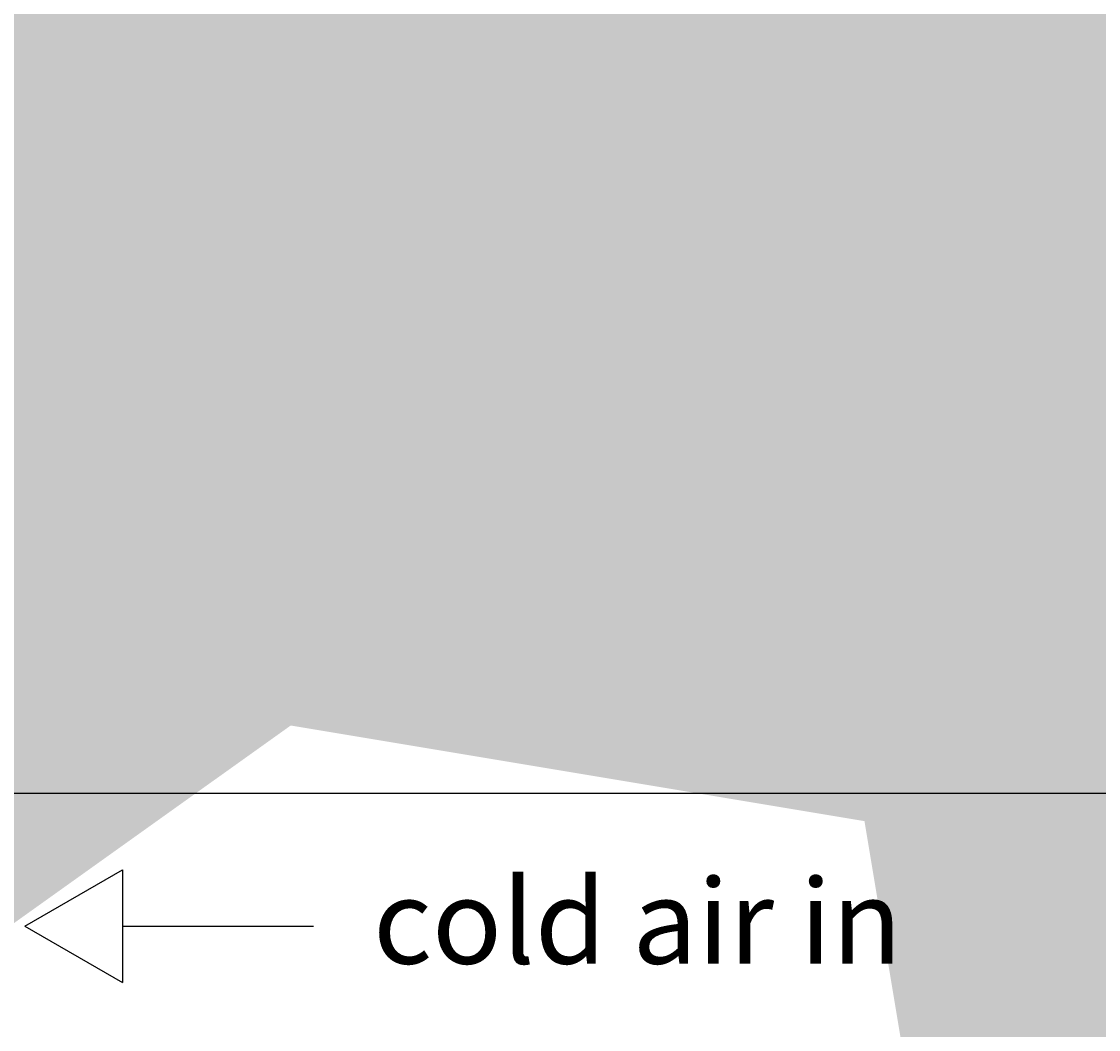
# Model space of a CAD drawing. Units: millimetres. Extents: x -22994 to 29398, y -19990 to 20176.
# Tile 121 of 135: x 245 to 296, y 165 to 213. Entities that reach past the tile are written whole.
import ezdxf

# ---------------------------------------------------------------- set-up
doc = ezdxf.new("R2010")
doc.units = ezdxf.units.MM
doc.header["$MEASUREMENT"] = 0
for name, color, linetype, lineweight in [('M-ANNO-SYMB', 7, 'Continuous', 25), ('M-ANNO-TEXT', 7, 'Continuous', 25), ('M-DIMS', 2, 'Continuous', 18)]:
    doc.layers.add(name, color=color, linetype=linetype, lineweight=lineweight)
doc.styles.get("Standard").update_dxf_attribs({"font": 'arial.ttf'})
doc.dimstyles.get("Standard").update_dxf_attribs({"dimtxt": 0.18, "dimasz": 10000, "dimexe": 0.18, "dimexo": 0.0625, "dimgap": 0.09, "dimtad": 0, "dimtih": 1, "dimtoh": 1, "dimdec": 0, "dimzin": 0, "dimdsep": 46, "dimtxsty": 'Standard', "dimcen": 0.09, "dimadec": 0, "dimazin": 0, "dimtfac": 1, "dimtdec": 0, "dimtofl": 0, "dimtmove": 0, "dimatfit": 3, "dimfxl": 1, "dimtolj": 1, "dimtzin": 0, "dimlwd": 30, "dimarcsym": 0})

# ---------------------------------------------------------------- blocks, each defined once
blk = doc.blocks.new('ARROW-FLOW')
for p, q in [((4.609, 5.322), (0, 2.661)), ((4.609, 5.322), (4.609, 0)), ((4.609, 0), (0, 2.661))]:
    blk.add_line(p, q)
blk = doc.blocks.new('*D2')
at = {"layer": 'Defpoints', "color": 0, "transparency": 16777216}
for p in [(6.677, 10.271), (290.852, 10.271), (290.852, -5.079)]:
    blk.add_point(p, dxfattribs=at)
at = {"layer": 'M-DIMS', "color": 0, "lineweight": -2, "transparency": 16777216}
for p, q in [((6.677, 10.209), (6.677, -5.259)), ((290.852, 10.209), (290.852, -5.259))]:
    blk.add_line(p, q, dxfattribs=at)
at = {"layer": 'M-DIMS', "color": 0, "lineweight": 30, "transparency": 16777216}
for p, q in [((-9993.323, -5.079), (-19993.323, -5.079)), ((10290.852, -5.079), (20290.852, -5.079))]:
    blk.add_line(p, q, dxfattribs=at)
at = {"layer": 'M-DIMS', "color": 0, "transparency": 16777216}
for points in [[(-9993.323, 1661.588), (-9993.323, -1671.745), (6.677, -5.079)], [(10290.852, 1661.588), (10290.852, -1671.745), (290.852, -5.079)]]:
    blk.add_solid(points, dxfattribs=at)
at = {"layer": 'M-DIMS', "color": 0, "transparency": 16777216, "insert": (148.765, -5.079), "char_height": 0.18, "attachment_point": 5}
blk.add_mtext('\\A1;284.2', dxfattribs=at)
blk = doc.blocks.new('*D3')
at = {"layer": 'Defpoints', "color": 0, "transparency": 16777216}
for p in [(110.265, 204.165), (110.265, 176.366), (95.833, 127.967)]:
    blk.add_point(p, dxfattribs=at)
at = {"layer": 'M-DIMS', "color": 0, "lineweight": 30, "transparency": 16777216}
for p, q in [((-9904.167, 204.165), (-19904.167, 204.165)), ((10110.265, 204.165), (20110.265, 204.165))]:
    blk.add_line(p, q, dxfattribs=at)
at = {"layer": 'M-DIMS', "color": 0, "lineweight": -2, "transparency": 16777216}
for p, q in [((95.833, 128.03), (95.833, 204.345)), ((110.265, 176.429), (110.265, 204.345))]:
    blk.add_line(p, q, dxfattribs=at)
at = {"layer": 'M-DIMS', "color": 0, "transparency": 16777216}
for points in [[(-9904.167, 1870.832), (-9904.167, -1462.501), (95.833, 204.165)], [(10110.265, 1870.832), (10110.265, -1462.501), (110.265, 204.165)]]:
    blk.add_solid(points, dxfattribs=at)
at = {"layer": 'M-DIMS', "color": 0, "transparency": 16777216, "insert": (103.049, 204.165), "char_height": 0.18, "attachment_point": 5}
blk.add_mtext('\\A1;14.432', dxfattribs=at)
blk = doc.blocks.new('*D4')
at = {"layer": 'Defpoints', "color": 0, "transparency": 16777216}
for p in [(116.265, 204.165), (110.265, 176.366), (116.265, 176.366)]:
    blk.add_point(p, dxfattribs=at)
at = {"layer": 'M-DIMS', "color": 0, "lineweight": 30, "transparency": 16777216}
for p, q in [((-9889.735, 204.165), (-19889.735, 204.165)), ((10116.265, 204.165), (20116.265, 204.165))]:
    blk.add_line(p, q, dxfattribs=at)
at = {"layer": 'M-DIMS', "color": 0, "lineweight": -2, "transparency": 16777216}
for p, q in [((110.265, 176.429), (110.265, 204.345)), ((116.265, 176.429), (116.265, 204.345))]:
    blk.add_line(p, q, dxfattribs=at)
at = {"layer": 'M-DIMS', "color": 0, "transparency": 16777216}
for points in [[(-9889.735, 1870.832), (-9889.735, -1462.501), (110.265, 204.165)], [(10116.265, 1870.832), (10116.265, -1462.501), (116.265, 204.165)]]:
    blk.add_solid(points, dxfattribs=at)
at = {"layer": 'M-DIMS', "color": 0, "transparency": 16777216, "insert": (113.265, 204.165), "char_height": 0.18, "attachment_point": 5}
blk.add_mtext('\\A1;6', dxfattribs=at)
blk = doc.blocks.new('*D5')
at = {"layer": 'Defpoints', "color": 0, "transparency": 16777216}
for p in [(181.265, 204.165), (116.265, 176.366), (181.265, 176.366)]:
    blk.add_point(p, dxfattribs=at)
at = {"layer": 'M-DIMS', "color": 0, "lineweight": 30, "transparency": 16777216}
for p, q in [((-9883.735, 204.165), (-19883.735, 204.165)), ((10181.265, 204.165), (20181.265, 204.165))]:
    blk.add_line(p, q, dxfattribs=at)
at = {"layer": 'M-DIMS', "color": 0, "lineweight": -2, "transparency": 16777216}
for p, q in [((116.265, 176.429), (116.265, 204.345)), ((181.265, 176.429), (181.265, 204.345))]:
    blk.add_line(p, q, dxfattribs=at)
at = {"layer": 'M-DIMS', "color": 0, "transparency": 16777216}
for points in [[(-9883.735, 1870.832), (-9883.735, -1462.501), (116.265, 204.165)], [(10181.265, 1870.832), (10181.265, -1462.501), (181.265, 204.165)]]:
    blk.add_solid(points, dxfattribs=at)
at = {"layer": 'M-DIMS', "color": 0, "transparency": 16777216, "insert": (148.765, 204.165), "char_height": 0.18, "attachment_point": 5}
blk.add_mtext('\\A1;65', dxfattribs=at)
blk = doc.blocks.new('*D6')
at = {"layer": 'Defpoints', "color": 0, "transparency": 16777216}
for p in [(187.265, 204.165), (181.265, 176.366), (187.265, 176.366)]:
    blk.add_point(p, dxfattribs=at)
at = {"layer": 'M-DIMS', "color": 0, "lineweight": 30, "transparency": 16777216}
for p, q in [((-9818.735, 204.165), (-19818.735, 204.165)), ((10187.265, 204.165), (20187.265, 204.165))]:
    blk.add_line(p, q, dxfattribs=at)
at = {"layer": 'M-DIMS', "color": 0, "lineweight": -2, "transparency": 16777216}
for p, q in [((181.265, 176.429), (181.265, 204.345)), ((187.265, 176.429), (187.265, 204.345))]:
    blk.add_line(p, q, dxfattribs=at)
at = {"layer": 'M-DIMS', "color": 0, "transparency": 16777216}
for points in [[(-9818.735, 1870.832), (-9818.735, -1462.501), (181.265, 204.165)], [(10187.265, 1870.832), (10187.265, -1462.501), (187.265, 204.165)]]:
    blk.add_solid(points, dxfattribs=at)
at = {"layer": 'M-DIMS', "color": 0, "transparency": 16777216, "insert": (184.265, 204.165), "char_height": 0.18, "attachment_point": 5}
blk.add_mtext('\\A1;6', dxfattribs=at)
blk = doc.blocks.new('*D7')
at = {"layer": 'Defpoints', "color": 0, "transparency": 16777216}
for p in [(201.697, 204.165), (187.265, 176.366), (201.697, 127.967)]:
    blk.add_point(p, dxfattribs=at)
at = {"layer": 'M-DIMS', "color": 0, "lineweight": 30, "transparency": 16777216}
for p, q in [((-9812.735, 204.165), (-19812.735, 204.165)), ((10201.697, 204.165), (20201.697, 204.165))]:
    blk.add_line(p, q, dxfattribs=at)
at = {"layer": 'M-DIMS', "color": 0, "lineweight": -2, "transparency": 16777216}
for p, q in [((187.265, 176.429), (187.265, 204.345)), ((201.697, 128.03), (201.697, 204.345))]:
    blk.add_line(p, q, dxfattribs=at)
at = {"layer": 'M-DIMS', "color": 0, "transparency": 16777216}
for points in [[(-9812.735, 1870.832), (-9812.735, -1462.501), (187.265, 204.165)], [(10201.697, 1870.832), (10201.697, -1462.501), (201.697, 204.165)]]:
    blk.add_solid(points, dxfattribs=at)
at = {"layer": 'M-DIMS', "color": 0, "transparency": 16777216, "insert": (194.481, 204.165), "char_height": 0.18, "attachment_point": 5}
blk.add_mtext('\\A1;14.432', dxfattribs=at)
blk = doc.blocks.new('*D8')
at = {"layer": 'Defpoints', "color": 0, "transparency": 16777216}
for p in [(227.648, 204.165), (227.648, 146.73), (201.697, 127.967)]:
    blk.add_point(p, dxfattribs=at)
at = {"layer": 'M-DIMS', "color": 0, "lineweight": 30, "transparency": 16777216}
for p, q in [((-9798.303, 204.165), (-19798.303, 204.165)), ((10227.648, 204.165), (20227.648, 204.165))]:
    blk.add_line(p, q, dxfattribs=at)
at = {"layer": 'M-DIMS', "color": 0, "lineweight": -2, "transparency": 16777216}
for p, q in [((201.697, 128.03), (201.697, 204.345)), ((227.648, 146.792), (227.648, 204.345))]:
    blk.add_line(p, q, dxfattribs=at)
at = {"layer": 'M-DIMS', "color": 0, "transparency": 16777216}
for points in [[(-9798.303, 1870.832), (-9798.303, -1462.501), (201.697, 204.165)], [(10227.648, 1870.832), (10227.648, -1462.501), (227.648, 204.165)]]:
    blk.add_solid(points, dxfattribs=at)
at = {"layer": 'M-DIMS', "color": 0, "transparency": 16777216, "insert": (214.673, 204.165), "char_height": 0.18, "attachment_point": 5}
blk.add_mtext('\\A1;25.95', dxfattribs=at)
blk = doc.blocks.new('*D9')
at = {"layer": 'Defpoints', "color": 0, "transparency": 16777216}
for p in [(187.265, 176.366), (306.202, 176.366), (290.852, 10.271)]:
    blk.add_point(p, dxfattribs=at)
at = {"layer": 'M-DIMS', "color": 0, "lineweight": 30, "transparency": 16777216}
for p, q in [((306.202, 10176.366), (306.202, 20176.366)), ((306.202, -9989.729), (306.202, -19989.729))]:
    blk.add_line(p, q, dxfattribs=at)
at = {"layer": 'M-DIMS', "color": 0, "lineweight": -2, "transparency": 16777216}
for p, q in [((187.327, 176.366), (306.382, 176.366)), ((290.915, 10.271), (306.382, 10.271))]:
    blk.add_line(p, q, dxfattribs=at)
at = {"layer": 'M-DIMS', "color": 0, "transparency": 16777216}
for points in [[(-1360.465, 10176.366), (1972.869, 10176.366), (306.202, 176.366)], [(-1360.465, -9989.729), (1972.869, -9989.729), (306.202, 10.271)]]:
    blk.add_solid(points, dxfattribs=at)
at = {"layer": 'M-DIMS', "color": 0, "transparency": 16777216, "insert": (306.202, 93.319), "char_height": 0.18, "attachment_point": 5}
blk.add_mtext('\\A1;166.1', dxfattribs=at)
blk = doc.blocks.new('*D10')
at = {"layer": 'Defpoints', "color": 0, "transparency": 16777216}
for p in [(125.65, 136.071), (133.346, 136.071), (133.346, -5.079)]:
    blk.add_point(p, dxfattribs=at)
at = {"layer": 'M-DIMS', "color": 0, "lineweight": -2, "transparency": 16777216}
for p, q in [((125.65, 136.009), (125.65, -5.259)), ((133.346, 136.009), (133.346, -5.259))]:
    blk.add_line(p, q, dxfattribs=at)
at = {"layer": 'M-DIMS', "color": 0, "lineweight": 30, "transparency": 16777216}
for p, q in [((-9874.35, -5.079), (-19874.35, -5.079)), ((10133.346, -5.079), (20133.346, -5.079))]:
    blk.add_line(p, q, dxfattribs=at)
at = {"layer": 'M-DIMS', "color": 0, "transparency": 16777216}
for points in [[(-9874.35, 1661.588), (-9874.35, -1671.745), (125.65, -5.079)], [(10133.346, 1661.588), (10133.346, -1671.745), (133.346, -5.079)]]:
    blk.add_solid(points, dxfattribs=at)
at = {"layer": 'M-DIMS', "color": 0, "transparency": 16777216, "insert": (129.498, -5.079), "char_height": 0.18, "attachment_point": 5}
blk.add_mtext('\\A1;7.696', dxfattribs=at)
blk = doc.blocks.new('*D11')
at = {"layer": 'Defpoints', "color": 0, "transparency": 16777216}
for p in [(133.346, 136.071), (135.65, 136.071), (135.65, -5.079)]:
    blk.add_point(p, dxfattribs=at)
at = {"layer": 'M-DIMS', "color": 0, "lineweight": -2, "transparency": 16777216}
for p, q in [((133.346, 136.009), (133.346, -5.259)), ((135.65, 136.009), (135.65, -5.259))]:
    blk.add_line(p, q, dxfattribs=at)
at = {"layer": 'M-DIMS', "color": 0, "lineweight": 30, "transparency": 16777216}
for p, q in [((-9866.654, -5.079), (-19866.654, -5.079)), ((10135.65, -5.079), (20135.65, -5.079))]:
    blk.add_line(p, q, dxfattribs=at)
at = {"layer": 'M-DIMS', "color": 0, "transparency": 16777216}
for points in [[(-9866.654, 1661.588), (-9866.654, -1671.745), (133.346, -5.079)], [(10135.65, 1661.588), (10135.65, -1671.745), (135.65, -5.079)]]:
    blk.add_solid(points, dxfattribs=at)
at = {"layer": 'M-DIMS', "color": 0, "transparency": 16777216, "insert": (134.498, -5.079), "char_height": 0.18, "attachment_point": 5}
blk.add_mtext('\\A1;2.304', dxfattribs=at)
blk = doc.blocks.new('*D12')
at = {"layer": 'Defpoints', "color": 0, "transparency": 16777216}
for p in [(135.65, 136.071), (145.65, 136.071), (145.65, -5.079)]:
    blk.add_point(p, dxfattribs=at)
at = {"layer": 'M-DIMS', "color": 0, "lineweight": -2, "transparency": 16777216}
for p, q in [((135.65, 136.009), (135.65, -5.259)), ((145.65, 136.009), (145.65, -5.259))]:
    blk.add_line(p, q, dxfattribs=at)
at = {"layer": 'M-DIMS', "color": 0, "lineweight": 30, "transparency": 16777216}
for p, q in [((-9864.35, -5.079), (-19864.35, -5.079)), ((10145.65, -5.079), (20145.65, -5.079))]:
    blk.add_line(p, q, dxfattribs=at)
at = {"layer": 'M-DIMS', "color": 0, "transparency": 16777216}
for points in [[(-9864.35, 1661.588), (-9864.35, -1671.745), (135.65, -5.079)], [(10145.65, 1661.588), (10145.65, -1671.745), (145.65, -5.079)]]:
    blk.add_solid(points, dxfattribs=at)
at = {"layer": 'M-DIMS', "color": 0, "transparency": 16777216, "insert": (140.65, -5.079), "char_height": 0.18, "attachment_point": 5}
blk.add_mtext('\\A1;10', dxfattribs=at)
blk = doc.blocks.new('*D13')
at = {"layer": 'Defpoints', "color": 0, "transparency": 16777216}
for p in [(145.65, 136.071), (155.65, 136.071), (155.65, -5.079)]:
    blk.add_point(p, dxfattribs=at)
at = {"layer": 'M-DIMS', "color": 0, "lineweight": -2, "transparency": 16777216}
for p, q in [((145.65, 136.009), (145.65, -5.259)), ((155.65, 136.009), (155.65, -5.259))]:
    blk.add_line(p, q, dxfattribs=at)
at = {"layer": 'M-DIMS', "color": 0, "lineweight": 30, "transparency": 16777216}
for p, q in [((-9854.35, -5.079), (-19854.35, -5.079)), ((10155.65, -5.079), (20155.65, -5.079))]:
    blk.add_line(p, q, dxfattribs=at)
at = {"layer": 'M-DIMS', "color": 0, "transparency": 16777216}
for points in [[(-9854.35, 1661.588), (-9854.35, -1671.745), (145.65, -5.079)], [(10155.65, 1661.588), (10155.65, -1671.745), (155.65, -5.079)]]:
    blk.add_solid(points, dxfattribs=at)
at = {"layer": 'M-DIMS', "color": 0, "transparency": 16777216, "insert": (150.65, -5.079), "char_height": 0.18, "attachment_point": 5}
blk.add_mtext('\\A1;10', dxfattribs=at)
blk = doc.blocks.new('*D14')
at = {"layer": 'Defpoints', "color": 0, "transparency": 16777216}
for p in [(155.65, 136.071), (165.65, 136.071), (165.65, -5.079)]:
    blk.add_point(p, dxfattribs=at)
at = {"layer": 'M-DIMS', "color": 0, "lineweight": -2, "transparency": 16777216}
for p, q in [((155.65, 136.009), (155.65, -5.259)), ((165.65, 136.009), (165.65, -5.259))]:
    blk.add_line(p, q, dxfattribs=at)
at = {"layer": 'M-DIMS', "color": 0, "lineweight": 30, "transparency": 16777216}
for p, q in [((-9844.35, -5.079), (-19844.35, -5.079)), ((10165.65, -5.079), (20165.65, -5.079))]:
    blk.add_line(p, q, dxfattribs=at)
at = {"layer": 'M-DIMS', "color": 0, "transparency": 16777216}
for points in [[(-9844.35, 1661.588), (-9844.35, -1671.745), (155.65, -5.079)], [(10165.65, 1661.588), (10165.65, -1671.745), (165.65, -5.079)]]:
    blk.add_solid(points, dxfattribs=at)
at = {"layer": 'M-DIMS', "color": 0, "transparency": 16777216, "insert": (160.65, -5.079), "char_height": 0.18, "attachment_point": 5}
blk.add_mtext('\\A1;10', dxfattribs=at)
blk = doc.blocks.new('*D15')
at = {"layer": 'Defpoints', "color": 0, "transparency": 16777216}
for p in [(173.346, 154.788), (173.346, 136.071), (306.202, 136.071)]:
    blk.add_point(p, dxfattribs=at)
at = {"layer": 'M-DIMS', "color": 0, "lineweight": 30, "transparency": 16777216}
for p, q in [((306.202, 10154.788), (306.202, 20154.788)), ((306.202, -9863.929), (306.202, -19863.929))]:
    blk.add_line(p, q, dxfattribs=at)
at = {"layer": 'M-DIMS', "color": 0, "lineweight": -2, "transparency": 16777216}
for p, q in [((173.408, 154.788), (306.382, 154.788)), ((173.408, 136.071), (306.382, 136.071))]:
    blk.add_line(p, q, dxfattribs=at)
at = {"layer": 'M-DIMS', "color": 0, "transparency": 16777216}
for points in [[(-1360.465, 10154.788), (1972.869, 10154.788), (306.202, 154.788)], [(-1360.465, -9863.929), (1972.869, -9863.929), (306.202, 136.071)]]:
    blk.add_solid(points, dxfattribs=at)
at = {"layer": 'M-DIMS', "color": 0, "transparency": 16777216, "insert": (306.202, 145.43), "char_height": 0.18, "attachment_point": 5}
blk.add_mtext('\\A1;18.717', dxfattribs=at)
blk = doc.blocks.new('*D16')
at = {"layer": 'Defpoints', "color": 0, "transparency": 16777216}
for p in [(120.17, 204.165), (110.466, 48.035), (120.17, 48.035)]:
    blk.add_point(p, dxfattribs=at)
at = {"layer": 'M-DIMS', "color": 0, "lineweight": 30, "transparency": 16777216}
for p, q in [((-9889.534, 204.165), (-19889.534, 204.165)), ((10120.17, 204.165), (20120.17, 204.165))]:
    blk.add_line(p, q, dxfattribs=at)
at = {"layer": 'M-DIMS', "color": 0, "lineweight": -2, "transparency": 16777216}
for p, q in [((110.466, 48.097), (110.466, 204.345)), ((120.17, 48.097), (120.17, 204.345))]:
    blk.add_line(p, q, dxfattribs=at)
at = {"layer": 'M-DIMS', "color": 0, "transparency": 16777216}
for points in [[(-9889.534, 1870.832), (-9889.534, -1462.501), (110.466, 204.165)], [(10120.17, 1870.832), (10120.17, -1462.501), (120.17, 204.165)]]:
    blk.add_solid(points, dxfattribs=at)
at = {"layer": 'M-DIMS', "color": 0, "transparency": 16777216, "insert": (115.318, 204.165), "char_height": 0.18, "attachment_point": 5}
blk.add_mtext('\\A1;9.704', dxfattribs=at)
blk = doc.blocks.new('*D17')
at = {"layer": 'Defpoints', "color": 0, "transparency": 16777216}
for p in [(126.17, 204.165), (120.17, 48.035), (126.17, 48.035)]:
    blk.add_point(p, dxfattribs=at)
at = {"layer": 'M-DIMS', "color": 0, "lineweight": 30, "transparency": 16777216}
for p, q in [((-9879.83, 204.165), (-19879.83, 204.165)), ((10126.17, 204.165), (20126.17, 204.165))]:
    blk.add_line(p, q, dxfattribs=at)
at = {"layer": 'M-DIMS', "color": 0, "lineweight": -2, "transparency": 16777216}
for p, q in [((120.17, 48.097), (120.17, 204.345)), ((126.17, 48.097), (126.17, 204.345))]:
    blk.add_line(p, q, dxfattribs=at)
at = {"layer": 'M-DIMS', "color": 0, "transparency": 16777216}
for points in [[(-9879.83, 1870.832), (-9879.83, -1462.501), (120.17, 204.165)], [(10126.17, 1870.832), (10126.17, -1462.501), (126.17, 204.165)]]:
    blk.add_solid(points, dxfattribs=at)
at = {"layer": 'M-DIMS', "color": 0, "transparency": 16777216, "insert": (123.17, 204.165), "char_height": 0.18, "attachment_point": 5}
blk.add_mtext('\\A1;6', dxfattribs=at)
blk = doc.blocks.new('*D18')
at = {"layer": 'Defpoints', "color": 0, "transparency": 16777216}
for p in [(132.17, 204.165), (126.17, 48.035), (132.17, 48.035)]:
    blk.add_point(p, dxfattribs=at)
at = {"layer": 'M-DIMS', "color": 0, "lineweight": 30, "transparency": 16777216}
for p, q in [((-9873.83, 204.165), (-19873.83, 204.165)), ((10132.17, 204.165), (20132.17, 204.165))]:
    blk.add_line(p, q, dxfattribs=at)
at = {"layer": 'M-DIMS', "color": 0, "lineweight": -2, "transparency": 16777216}
for p, q in [((126.17, 48.097), (126.17, 204.345)), ((132.17, 48.097), (132.17, 204.345))]:
    blk.add_line(p, q, dxfattribs=at)
at = {"layer": 'M-DIMS', "color": 0, "transparency": 16777216}
for points in [[(-9873.83, 1870.832), (-9873.83, -1462.501), (126.17, 204.165)], [(10132.17, 1870.832), (10132.17, -1462.501), (132.17, 204.165)]]:
    blk.add_solid(points, dxfattribs=at)
at = {"layer": 'M-DIMS', "color": 0, "transparency": 16777216, "insert": (129.17, 204.165), "char_height": 0.18, "attachment_point": 5}
blk.add_mtext('\\A1;6', dxfattribs=at)
blk = doc.blocks.new('*D19')
at = {"layer": 'Defpoints', "color": 0, "transparency": 16777216}
for p in [(138.17, 204.165), (132.17, 48.035), (138.17, 48.035)]:
    blk.add_point(p, dxfattribs=at)
at = {"layer": 'M-DIMS', "color": 0, "lineweight": 30, "transparency": 16777216}
for p, q in [((-9867.83, 204.165), (-19867.83, 204.165)), ((10138.17, 204.165), (20138.17, 204.165))]:
    blk.add_line(p, q, dxfattribs=at)
at = {"layer": 'M-DIMS', "color": 0, "lineweight": -2, "transparency": 16777216}
for p, q in [((132.17, 48.097), (132.17, 204.345)), ((138.17, 48.097), (138.17, 204.345))]:
    blk.add_line(p, q, dxfattribs=at)
at = {"layer": 'M-DIMS', "color": 0, "transparency": 16777216}
for points in [[(-9867.83, 1870.832), (-9867.83, -1462.501), (132.17, 204.165)], [(10138.17, 1870.832), (10138.17, -1462.501), (138.17, 204.165)]]:
    blk.add_solid(points, dxfattribs=at)
at = {"layer": 'M-DIMS', "color": 0, "transparency": 16777216, "insert": (135.17, 204.165), "char_height": 0.18, "attachment_point": 5}
blk.add_mtext('\\A1;6', dxfattribs=at)
blk = doc.blocks.new('*D20')
at = {"layer": 'Defpoints', "color": 0, "transparency": 16777216}
for p in [(144.17, 204.165), (138.17, 48.035), (144.17, 48.035)]:
    blk.add_point(p, dxfattribs=at)
at = {"layer": 'M-DIMS', "color": 0, "lineweight": 30, "transparency": 16777216}
for p, q in [((-9861.83, 204.165), (-19861.83, 204.165)), ((10144.17, 204.165), (20144.17, 204.165))]:
    blk.add_line(p, q, dxfattribs=at)
at = {"layer": 'M-DIMS', "color": 0, "lineweight": -2, "transparency": 16777216}
for p, q in [((138.17, 48.097), (138.17, 204.345)), ((144.17, 48.097), (144.17, 204.345))]:
    blk.add_line(p, q, dxfattribs=at)
at = {"layer": 'M-DIMS', "color": 0, "transparency": 16777216}
for points in [[(-9861.83, 1870.832), (-9861.83, -1462.501), (138.17, 204.165)], [(10144.17, 1870.832), (10144.17, -1462.501), (144.17, 204.165)]]:
    blk.add_solid(points, dxfattribs=at)
at = {"layer": 'M-DIMS', "color": 0, "transparency": 16777216, "insert": (141.17, 204.165), "char_height": 0.18, "attachment_point": 5}
blk.add_mtext('\\A1;6', dxfattribs=at)
blk = doc.blocks.new('*D21')
at = {"layer": 'Defpoints', "color": 0, "transparency": 16777216}
for p in [(149.116, 204.165), (144.17, 48.035), (149.116, 48.035)]:
    blk.add_point(p, dxfattribs=at)
at = {"layer": 'M-DIMS', "color": 0, "lineweight": 30, "transparency": 16777216}
for p, q in [((-9855.83, 204.165), (-19855.83, 204.165)), ((10149.116, 204.165), (20149.116, 204.165))]:
    blk.add_line(p, q, dxfattribs=at)
at = {"layer": 'M-DIMS', "color": 0, "lineweight": -2, "transparency": 16777216}
for p, q in [((144.17, 48.097), (144.17, 204.345)), ((149.116, 48.097), (149.116, 204.345))]:
    blk.add_line(p, q, dxfattribs=at)
at = {"layer": 'M-DIMS', "color": 0, "transparency": 16777216}
for points in [[(-9855.83, 1870.832), (-9855.83, -1462.501), (144.17, 204.165)], [(10149.116, 1870.832), (10149.116, -1462.501), (149.116, 204.165)]]:
    blk.add_solid(points, dxfattribs=at)
at = {"layer": 'M-DIMS', "color": 0, "transparency": 16777216, "insert": (146.643, 204.165), "char_height": 0.18, "attachment_point": 5}
blk.add_mtext('\\A1;4.945', dxfattribs=at)
blk = doc.blocks.new('*D22')
at = {"layer": 'Defpoints', "color": 0, "transparency": 16777216}
for p in [(149.116, 30.99), (155.116, 30.99), (155.116, -5.079)]:
    blk.add_point(p, dxfattribs=at)
at = {"layer": 'M-DIMS', "color": 0, "lineweight": -2, "transparency": 16777216}
for p, q in [((149.116, 30.927), (149.116, -5.259)), ((155.116, 30.927), (155.116, -5.259))]:
    blk.add_line(p, q, dxfattribs=at)
at = {"layer": 'M-DIMS', "color": 0, "lineweight": 30, "transparency": 16777216}
for p, q in [((-9850.884, -5.079), (-19850.884, -5.079)), ((10155.116, -5.079), (20155.116, -5.079))]:
    blk.add_line(p, q, dxfattribs=at)
at = {"layer": 'M-DIMS', "color": 0, "transparency": 16777216}
for points in [[(-9850.884, 1661.588), (-9850.884, -1671.745), (149.116, -5.079)], [(10155.116, 1661.588), (10155.116, -1671.745), (155.116, -5.079)]]:
    blk.add_solid(points, dxfattribs=at)
at = {"layer": 'M-DIMS', "color": 0, "transparency": 16777216, "insert": (152.116, -5.079), "char_height": 0.18, "attachment_point": 5}
blk.add_mtext('\\A1;6', dxfattribs=at)
blk = doc.blocks.new('*D23')
at = {"layer": 'Defpoints', "color": 0, "transparency": 16777216}
for p in [(155.116, 30.99), (161.116, 30.99), (161.116, -5.079)]:
    blk.add_point(p, dxfattribs=at)
at = {"layer": 'M-DIMS', "color": 0, "lineweight": -2, "transparency": 16777216}
for p, q in [((155.116, 30.927), (155.116, -5.259)), ((161.116, 30.927), (161.116, -5.259))]:
    blk.add_line(p, q, dxfattribs=at)
at = {"layer": 'M-DIMS', "color": 0, "lineweight": 30, "transparency": 16777216}
for p, q in [((-9844.884, -5.079), (-19844.884, -5.079)), ((10161.116, -5.079), (20161.116, -5.079))]:
    blk.add_line(p, q, dxfattribs=at)
at = {"layer": 'M-DIMS', "color": 0, "transparency": 16777216}
for points in [[(-9844.884, 1661.588), (-9844.884, -1671.745), (155.116, -5.079)], [(10161.116, 1661.588), (10161.116, -1671.745), (161.116, -5.079)]]:
    blk.add_solid(points, dxfattribs=at)
at = {"layer": 'M-DIMS', "color": 0, "transparency": 16777216, "insert": (158.116, -5.079), "char_height": 0.18, "attachment_point": 5}
blk.add_mtext('\\A1;6', dxfattribs=at)
blk = doc.blocks.new('*D24')
at = {"layer": 'Defpoints', "color": 0, "transparency": 16777216}
for p in [(161.116, 30.99), (166.439, 30.99), (166.439, -5.079)]:
    blk.add_point(p, dxfattribs=at)
at = {"layer": 'M-DIMS', "color": 0, "lineweight": -2, "transparency": 16777216}
for p, q in [((161.116, 30.927), (161.116, -5.259)), ((166.439, 30.927), (166.439, -5.259))]:
    blk.add_line(p, q, dxfattribs=at)
at = {"layer": 'M-DIMS', "color": 0, "lineweight": 30, "transparency": 16777216}
for p, q in [((-9838.884, -5.079), (-19838.884, -5.079)), ((10166.439, -5.079), (20166.439, -5.079))]:
    blk.add_line(p, q, dxfattribs=at)
at = {"layer": 'M-DIMS', "color": 0, "transparency": 16777216}
for points in [[(-9838.884, 1661.588), (-9838.884, -1671.745), (161.116, -5.079)], [(10166.439, 1661.588), (10166.439, -1671.745), (166.439, -5.079)]]:
    blk.add_solid(points, dxfattribs=at)
at = {"layer": 'M-DIMS', "color": 0, "transparency": 16777216, "insert": (163.777, -5.079), "char_height": 0.18, "attachment_point": 5}
blk.add_mtext('\\A1;5.323', dxfattribs=at)
blk = doc.blocks.new('*D25')
at = {"layer": 'Defpoints', "color": 0, "transparency": 16777216}
for p in [(166.439, 30.99), (172.439, 30.99), (172.439, -5.079)]:
    blk.add_point(p, dxfattribs=at)
at = {"layer": 'M-DIMS', "color": 0, "lineweight": -2, "transparency": 16777216}
for p, q in [((166.439, 30.927), (166.439, -5.259)), ((172.439, 30.927), (172.439, -5.259))]:
    blk.add_line(p, q, dxfattribs=at)
at = {"layer": 'M-DIMS', "color": 0, "lineweight": 30, "transparency": 16777216}
for p, q in [((-9833.561, -5.079), (-19833.561, -5.079)), ((10172.439, -5.079), (20172.439, -5.079))]:
    blk.add_line(p, q, dxfattribs=at)
at = {"layer": 'M-DIMS', "color": 0, "transparency": 16777216}
for points in [[(-9833.561, 1661.588), (-9833.561, -1671.745), (166.439, -5.079)], [(10172.439, 1661.588), (10172.439, -1671.745), (172.439, -5.079)]]:
    blk.add_solid(points, dxfattribs=at)
at = {"layer": 'M-DIMS', "color": 0, "transparency": 16777216, "insert": (169.439, -5.079), "char_height": 0.18, "attachment_point": 5}
blk.add_mtext('\\A1;6', dxfattribs=at)
blk = doc.blocks.new('*D26')
at = {"layer": 'Defpoints', "color": 0, "transparency": 16777216}
for p in [(172.439, 30.99), (178.439, 30.99), (178.439, -5.079)]:
    blk.add_point(p, dxfattribs=at)
at = {"layer": 'M-DIMS', "color": 0, "lineweight": -2, "transparency": 16777216}
for p, q in [((172.439, 30.927), (172.439, -5.259)), ((178.439, 30.927), (178.439, -5.259))]:
    blk.add_line(p, q, dxfattribs=at)
at = {"layer": 'M-DIMS', "color": 0, "lineweight": 30, "transparency": 16777216}
for p, q in [((-9827.561, -5.079), (-19827.561, -5.079)), ((10178.439, -5.079), (20178.439, -5.079))]:
    blk.add_line(p, q, dxfattribs=at)
at = {"layer": 'M-DIMS', "color": 0, "transparency": 16777216}
for points in [[(-9827.561, 1661.588), (-9827.561, -1671.745), (172.439, -5.079)], [(10178.439, 1661.588), (10178.439, -1671.745), (178.439, -5.079)]]:
    blk.add_solid(points, dxfattribs=at)
at = {"layer": 'M-DIMS', "color": 0, "transparency": 16777216, "insert": (175.439, -5.079), "char_height": 0.18, "attachment_point": 5}
blk.add_mtext('\\A1;6', dxfattribs=at)
blk = doc.blocks.new('*D27')
at = {"layer": 'Defpoints', "color": 0, "transparency": 16777216}
for p in [(178.439, 30.99), (188.117, 30.99), (188.117, -5.079)]:
    blk.add_point(p, dxfattribs=at)
at = {"layer": 'M-DIMS', "color": 0, "lineweight": -2, "transparency": 16777216}
for p, q in [((178.439, 30.927), (178.439, -5.259)), ((188.117, 30.927), (188.117, -5.259))]:
    blk.add_line(p, q, dxfattribs=at)
at = {"layer": 'M-DIMS', "color": 0, "lineweight": 30, "transparency": 16777216}
for p, q in [((-9821.561, -5.079), (-19821.561, -5.079)), ((10188.117, -5.079), (20188.117, -5.079))]:
    blk.add_line(p, q, dxfattribs=at)
at = {"layer": 'M-DIMS', "color": 0, "transparency": 16777216}
for points in [[(-9821.561, 1661.588), (-9821.561, -1671.745), (178.439, -5.079)], [(10188.117, 1661.588), (10188.117, -1671.745), (188.117, -5.079)]]:
    blk.add_solid(points, dxfattribs=at)
at = {"layer": 'M-DIMS', "color": 0, "transparency": 16777216, "insert": (183.278, -5.079), "char_height": 0.18, "attachment_point": 5}
blk.add_mtext('\\A1;9.679', dxfattribs=at)
blk = doc.blocks.new('*D28')
at = {"layer": 'Defpoints', "color": 0, "transparency": 16777216}
for p in [(188.117, 48.035), (306.202, 48.035), (188.117, 30.99)]:
    blk.add_point(p, dxfattribs=at)
at = {"layer": 'M-DIMS', "color": 0, "lineweight": 30, "transparency": 16777216}
for p, q in [((306.202, 10048.035), (306.202, 20048.035)), ((306.202, -9969.01), (306.202, -19969.01))]:
    blk.add_line(p, q, dxfattribs=at)
at = {"layer": 'M-DIMS', "color": 0, "lineweight": -2, "transparency": 16777216}
for p, q in [((188.18, 48.035), (306.382, 48.035)), ((188.18, 30.99), (306.382, 30.99))]:
    blk.add_line(p, q, dxfattribs=at)
at = {"layer": 'M-DIMS', "color": 0, "transparency": 16777216}
for points in [[(-1360.465, 10048.035), (1972.869, 10048.035), (306.202, 48.035)], [(-1360.465, -9969.01), (1972.869, -9969.01), (306.202, 30.99)]]:
    blk.add_solid(points, dxfattribs=at)
at = {"layer": 'M-DIMS', "color": 0, "transparency": 16777216, "insert": (306.202, 39.512), "char_height": 0.18, "attachment_point": 5}
blk.add_mtext('\\A1;17.045', dxfattribs=at)
blk = doc.blocks.new('*D29')
at = {"layer": 'Defpoints', "color": 0, "transparency": 16777216}
for p in [(36.801, 80.045), (64.03, 80.045)]:
    blk.add_point(p, dxfattribs=at)
at = {"layer": 'M-DIMS', "color": 0, "lineweight": -2, "transparency": 16777216}
for p, q in [((50.325, 80.045), (50.505, 80.045)), ((50.415, 79.955), (50.415, 80.135))]:
    blk.add_line(p, q, dxfattribs=at)
at = {"layer": 'M-DIMS', "color": 0, "lineweight": 30, "transparency": 16777216}
blk.add_line((20064.03, 80.03), (10064.03, 80.038), dxfattribs=at)
at = {"layer": 'M-DIMS', "color": 0, "transparency": 16777216}
blk.add_solid([(10064.031, 1746.704), (10064.028, -1586.629), (64.03, 80.045)], dxfattribs=at)
at = {"layer": 'M-DIMS', "color": 0, "transparency": 16777216, "insert": (20064.521, 80.03), "char_height": 0.18, "attachment_point": 5}
blk.add_mtext('\\A1;∅27.23', dxfattribs=at)
blk = doc.blocks.new('*D30')
at = {"layer": 'Defpoints', "color": 0, "transparency": 16777216}
for p in [(216.315, 146.729), (238.982, 146.73)]:
    blk.add_point(p, dxfattribs=at)
at = {"layer": 'M-DIMS', "color": 0, "lineweight": 30, "transparency": 16777216}
blk.add_line((20238.982, 147.496), (10238.982, 147.113), dxfattribs=at)
at = {"layer": 'M-DIMS', "color": 0, "lineweight": -2, "transparency": 16777216}
for p, q in [((227.558, 146.73), (227.738, 146.73)), ((227.648, 146.64), (227.648, 146.82))]:
    blk.add_line(p, q, dxfattribs=at)
at = {"layer": 'M-DIMS', "color": 0, "transparency": 16777216}
blk.add_solid([(10238.918, 1813.78), (10239.046, -1519.554), (238.982, 146.73)], dxfattribs=at)
at = {"layer": 'M-DIMS', "color": 0, "transparency": 16777216, "insert": (20239.544, 147.496), "char_height": 0.18, "attachment_point": 5}
blk.add_mtext('\\A1;∅22.667', dxfattribs=at)
blk = doc.blocks.new('*D31')
at = {"layer": 'Defpoints', "color": 0, "transparency": 16777216}
for p in [(223.164, 146.729), (232.133, 146.73)]:
    blk.add_point(p, dxfattribs=at)
at = {"layer": 'M-DIMS', "color": 0, "lineweight": 30, "transparency": 16777216}
blk.add_line((20232.133, 148.666), (10232.133, 147.698), dxfattribs=at)
at = {"layer": 'M-DIMS', "color": 0, "lineweight": -2, "transparency": 16777216}
for p, q in [((227.558, 146.73), (227.738, 146.73)), ((227.648, 146.64), (227.648, 146.82))]:
    blk.add_line(p, q, dxfattribs=at)
at = {"layer": 'M-DIMS', "color": 0, "transparency": 16777216}
blk.add_solid([(10231.971, 1814.364), (10232.294, -1518.969), (232.133, 146.73)], dxfattribs=at)
at = {"layer": 'M-DIMS', "color": 0, "transparency": 16777216, "insert": (20232.625, 148.666), "char_height": 0.18, "attachment_point": 5}
blk.add_mtext('\\A1;∅8.969', dxfattribs=at)
blk = doc.blocks.new('*D34')
at = {"layer": 'Defpoints', "color": 0, "transparency": 16777216}
for p in [(178.58, 122.895), (176.812, 121.128)]:
    blk.add_point(p, dxfattribs=at)
at = {"layer": 'M-DIMS', "color": 0, "lineweight": 30, "transparency": 16777216}
for p, q in [((14322.436, 14263.311), (7250.508, 7193.103)), ((24322.436, 14263.311), (14322.436, 14263.311))]:
    blk.add_line(p, q, dxfattribs=at)
at = {"layer": 'M-DIMS', "color": 0, "lineweight": -2, "transparency": 16777216}
for p, q in [((176.722, 121.128), (176.902, 121.128)), ((176.812, 121.038), (176.812, 121.218))]:
    blk.add_line(p, q, dxfattribs=at)
at = {"layer": 'M-DIMS', "color": 0, "transparency": 16777216}
blk.add_solid([(6072.14, 8371.758), (8428.876, 6014.448), (178.58, 122.895)], dxfattribs=at)
at = {"layer": 'M-DIMS', "color": 0, "transparency": 16777216, "insert": (24322.97, 14263.311), "char_height": 0.18, "attachment_point": 5}
blk.add_mtext('\\A1;6X R2.5', dxfattribs=at)
blk = doc.blocks.new('*D36')
at = {"layer": 'Defpoints', "color": 0, "transparency": 16777216}
for p in [(46.39, 31.303), (46.387, 26.593)]:
    blk.add_point(p, dxfattribs=at)
at = {"layer": 'M-DIMS', "color": 0, "lineweight": 30, "transparency": 16777216}
for p, q in [((57.15, 20031.301), (51.77, 10031.302)), ((10057.15, 20031.301), (57.15, 20031.301))]:
    blk.add_line(p, q, dxfattribs=at)
at = {"layer": 'M-DIMS', "color": 0, "lineweight": -2, "transparency": 16777216}
for p, q in [((46.389, 28.858), (46.389, 29.038)), ((46.299, 28.948), (46.479, 28.948))]:
    blk.add_line(p, q, dxfattribs=at)
at = {"layer": 'M-DIMS', "color": 0, "transparency": 16777216}
blk.add_solid([(-1614.896, 10032.199), (1718.436, 10030.405), (46.39, 31.303)], dxfattribs=at)
at = {"layer": 'M-DIMS', "color": 0, "transparency": 16777216, "insert": (10057.554, 20031.301), "char_height": 0.18, "attachment_point": 5}
blk.add_mtext('\\A1;∅4.71', dxfattribs=at)
blk = doc.blocks.new('*D37')
at = {"layer": 'Defpoints', "color": 0, "transparency": 16777216}
for p in [(54.834, 118.615), (59.494, 118.614)]:
    blk.add_point(p, dxfattribs=at)
at = {"layer": 'M-DIMS', "color": 0, "lineweight": -2, "transparency": 16777216}
for p, q in [((57.074, 118.614), (57.254, 118.614)), ((57.164, 118.524), (57.164, 118.704))]:
    blk.add_line(p, q, dxfattribs=at)
at = {"layer": 'M-DIMS', "color": 0, "lineweight": 30, "transparency": 16777216}
blk.add_line((20059.493, 116.253), (10059.494, 117.434), dxfattribs=at)
at = {"layer": 'M-DIMS', "color": 0, "transparency": 16777216}
blk.add_solid([(10059.69, 1784.1), (10059.297, -1549.233), (59.494, 118.614)], dxfattribs=at)
at = {"layer": 'M-DIMS', "color": 0, "transparency": 16777216, "insert": (20059.985, 116.253), "char_height": 0.18, "attachment_point": 5}
blk.add_mtext('\\A1;∅4.659', dxfattribs=at)

msp = doc.modelspace()

# ---------------------------------------------------------------- linework, layer by layer
at = {"layer": 'M-ANNO-SYMB'}
msp.add_line((249.9748, 170.0688), (259.0037, 170.0688), dxfattribs=at)

# ---------------------------------------------------------------- block references
at = {"layer": 'M-ANNO-SYMB', "rotation": 119.9999999999995}
msp.add_blockref('ARROW-FLOW', (252.2794, 168.7383), dxfattribs=at)

# ---------------------------------------------------------------- texts
at = {"layer": 'M-ANNO-TEXT', "insert": (261.8199, 172.2997), "char_height": 4, "attachment_point": 1}
msp.add_mtext_dynamic_manual_height_columns('cold air in', width=33.54165, gutter_width=1, heights=[0], dxfattribs=at)

# ---------------------------------------------------------------- dimensions: what is measured, and where the dimension line sits
at = {"layer": 'M-DIMS'}
for base, p1, p2, override, picture, middle in [((306.202, 176.3662), (290.852, 10.2713), (187.2647, 176.3662), {"dimdec": 1, "dimlfac": 1, "dimrnd": 0, "dimzin": 0, "dimdsep": 46, "dimlunit": 2}, '*D9', (306.202, 93.3187)), ((306.202, 136.0713), (173.3459, 154.788), (173.3459, 136.0713), {"dimdec": 3, "dimlfac": 1, "dimrnd": 0, "dimzin": 0, "dimdsep": 46, "dimlunit": 2}, '*D15', (306.202, 145.4297)), ((306.202, 48.0349), (188.1175, 30.9895), (188.1175, 48.0349), {"dimdec": 3, "dimlfac": 1, "dimrnd": 0, "dimzin": 0, "dimdsep": 46, "dimlunit": 2}, '*D28', (306.202, 39.5122))]:
    dim = msp.add_linear_dim(base=base, p1=p1, p2=p2, angle=90, dimstyle='Standard', override=override, dxfattribs=at)
    dim.commit()
    dim.dimension.update_dxf_attribs({"geometry": picture, "text_midpoint": middle})
for p1, p2, override, picture, middle in [((46.3875, 26.5934), (46.39, 31.3035), {"dimdec": 2, "dimlfac": 1, "dimrnd": 0, "dimzin": 0, "dimdsep": 46, "dimlunit": 2}, '*D36', (10057.5542, 20031.3006)), ((223.1641, 146.7291), (232.1328, 146.73), {"dimdec": 3, "dimlfac": 1, "dimrnd": 0, "dimzin": 0, "dimdsep": 46, "dimlunit": 2}, '*D31', (20232.1327, 148.6656)), ((216.3148, 146.7291), (238.9821, 146.73), {"dimdec": 3, "dimlfac": 1, "dimrnd": 0, "dimzin": 0, "dimdsep": 46, "dimlunit": 2}, '*D30', (20238.9821, 147.4959))]:
    dim = msp.add_diameter_dim_2p(p1=p1, p2=p2, dimstyle='Standard', override=override, dxfattribs=at)
    dim.commit()
    dim.dimension.update_dxf_attribs({"geometry": picture, "text_midpoint": middle, "dimtype": 163})
dim = msp.add_radius_dim(center=(176.8123, 121.1277), mpoint=(178.5802, 122.8952), text='6X <>', dimstyle='Standard', override={"dimdec": 1, "dimlfac": 1, "dimrnd": 0, "dimzin": 0, "dimdsep": 46, "dimlunit": 2}, dxfattribs=at)
dim.commit()
dim.dimension.update_dxf_attribs({"geometry": '*D34', "text_midpoint": (24322.9703, 14263.3108)})
for base, p1, p2, override, picture, middle in [((110.2647, 204.1654), (95.8327, 127.967), (110.2647, 176.3662), {"dimdec": 3, "dimlfac": 1, "dimrnd": 0, "dimzin": 0, "dimdsep": 46, "dimlunit": 2}, '*D3', (103.0487, 204.1654)), ((116.2647, 204.1654), (110.2647, 176.3662), (116.2647, 176.3662), {"dimdec": 0, "dimlfac": 1, "dimrnd": 0, "dimzin": 0, "dimdsep": 46, "dimlunit": 2}, '*D4', (113.2647, 204.1654)), ((120.1702, 204.1654), (110.4658, 48.0349), (120.1702, 48.0349), {"dimdec": 3, "dimlfac": 1, "dimrnd": 0, "dimzin": 0, "dimdsep": 46, "dimlunit": 2}, '*D16', (115.318, 204.1654)), ((181.2647, 204.1654), (116.2647, 176.3662), (181.2647, 176.3662), {"dimdec": 0, "dimlfac": 1, "dimrnd": 0, "dimzin": 0, "dimdsep": 46, "dimlunit": 2}, '*D5', (148.7647, 204.1654)), ((126.1702, 204.1654), (120.1702, 48.0349), (126.1702, 48.0349), {"dimdec": 0, "dimlfac": 1, "dimrnd": 0, "dimzin": 0, "dimdsep": 46, "dimlunit": 2}, '*D17', (123.1702, 204.1654)), ((132.1702, 204.1654), (126.1702, 48.0349), (132.1702, 48.0349), {"dimdec": 0, "dimlfac": 1, "dimrnd": 0, "dimzin": 0, "dimdsep": 46, "dimlunit": 2}, '*D18', (129.1702, 204.1654)), ((138.1702, 204.1654), (132.1702, 48.0349), (138.1702, 48.0349), {"dimdec": 0, "dimlfac": 1, "dimrnd": 0, "dimzin": 0, "dimdsep": 46, "dimlunit": 2}, '*D19', (135.1702, 204.1654)), ((144.1702, 204.1654), (138.1702, 48.0349), (144.1702, 48.0349), {"dimdec": 0, "dimlfac": 1, "dimrnd": 0, "dimzin": 0, "dimdsep": 46, "dimlunit": 2}, '*D20', (141.1702, 204.1654)), ((149.11567, 204.16539), (144.17023, 48.03494), (149.11567, 48.03494), {"dimdec": 3, "dimlfac": 1, "dimrnd": 0, "dimzin": 0, "dimdsep": 46, "dimlunit": 2}, '*D21', (146.64295, 204.16539)), ((187.2647, 204.1654), (181.2647, 176.3662), (187.2647, 176.3662), {"dimdec": 0, "dimlfac": 1, "dimrnd": 0, "dimzin": 0, "dimdsep": 46, "dimlunit": 2}, '*D6', (184.2647, 204.1654)), ((201.6967, 204.1654), (187.2647, 176.3662), (201.6967, 127.967), {"dimdec": 3, "dimlfac": 1, "dimrnd": 0, "dimzin": 0, "dimdsep": 46, "dimlunit": 2}, '*D7', (194.4807, 204.1654)), ((227.6485, 204.1654), (201.6967, 127.967), (227.6485, 146.7296), {"dimdec": 2, "dimlfac": 1, "dimrnd": 0, "dimzin": 0, "dimdsep": 46, "dimlunit": 2}, '*D8', (214.6726, 204.1654)), ((290.852, -5.0787), (6.6773, 10.2713), (290.852, 10.2713), {"dimdec": 1, "dimlfac": 1, "dimrnd": 0, "dimzin": 0, "dimdsep": 46, "dimlunit": 2}, '*D2', (148.7647, -5.0787)), ((133.3459, -5.0787), (125.6498, 136.0713), (133.3459, 136.0713), {"dimdec": 3, "dimlfac": 1, "dimrnd": 0, "dimzin": 0, "dimdsep": 46, "dimlunit": 2}, '*D10', (129.4978, -5.0787)), ((135.6498, -5.0787), (133.3459, 136.0713), (135.6498, 136.0713), {"dimdec": 3, "dimlfac": 1, "dimrnd": 0, "dimzin": 0, "dimdsep": 46, "dimlunit": 2}, '*D11', (134.4978, -5.0787)), ((145.6498, -5.0787), (135.6498, 136.0713), (145.6498, 136.0713), {"dimdec": 0, "dimlfac": 1, "dimrnd": 0, "dimzin": 0, "dimdsep": 46, "dimlunit": 2}, '*D12', (140.6498, -5.0787)), ((155.6498, -5.0787), (145.6498, 136.0713), (155.6498, 136.0713), {"dimdec": 0, "dimlfac": 1, "dimrnd": 0, "dimzin": 0, "dimdsep": 46, "dimlunit": 2}, '*D13', (150.6498, -5.0787)), ((155.1157, -5.0787), (149.1157, 30.9895), (155.1157, 30.9895), {"dimdec": 0, "dimlfac": 1, "dimrnd": 0, "dimzin": 0, "dimdsep": 46, "dimlunit": 2}, '*D22', (152.1157, -5.0787)), ((161.1157, -5.0787), (155.1157, 30.9895), (161.1157, 30.9895), {"dimdec": 0, "dimlfac": 1, "dimrnd": 0, "dimzin": 0, "dimdsep": 46, "dimlunit": 2}, '*D23', (158.1157, -5.0787)), ((165.6498, -5.0787), (155.6498, 136.0713), (165.6498, 136.0713), {"dimdec": 0, "dimlfac": 1, "dimrnd": 0, "dimzin": 0, "dimdsep": 46, "dimlunit": 2}, '*D14', (160.6498, -5.0787)), ((166.4387, -5.0787), (161.1157, 30.9895), (166.4387, 30.9895), {"dimdec": 3, "dimlfac": 1, "dimrnd": 0, "dimzin": 0, "dimdsep": 46, "dimlunit": 2}, '*D24', (163.7772, -5.0787)), ((172.4387, -5.0787), (166.4387, 30.9895), (172.4387, 30.9895), {"dimdec": 0, "dimlfac": 1, "dimrnd": 0, "dimzin": 0, "dimdsep": 46, "dimlunit": 2}, '*D25', (169.4387, -5.0787)), ((178.4387, -5.0787), (172.4387, 30.9895), (178.4387, 30.9895), {"dimdec": 0, "dimlfac": 1, "dimrnd": 0, "dimzin": 0, "dimdsep": 46, "dimlunit": 2}, '*D26', (175.4387, -5.0787)), ((188.1175, -5.0787), (178.4387, 30.9895), (188.1175, 30.9895), {"dimdec": 3, "dimlfac": 1, "dimrnd": 0, "dimzin": 0, "dimdsep": 46, "dimlunit": 2}, '*D27', (183.2781, -5.0787))]:
    dim = msp.add_linear_dim(base=base, p1=p1, p2=p2, dimstyle='Standard', override=override, dxfattribs=at)
    dim.commit()
    dim.dimension.update_dxf_attribs({"geometry": picture, "text_midpoint": middle})
for p1, p2, override, picture, middle in [((54.8343, 118.6145), (59.4936, 118.614), {"dimdec": 3, "dimlfac": 1, "dimrnd": 0, "dimzin": 0, "dimdsep": 46, "dimlunit": 2}, '*D37', (20059.4934, 116.2531)), ((36.8006, 80.045), (64.0296, 80.045), {"dimdec": 2, "dimlfac": 1, "dimrnd": 0, "dimzin": 0, "dimdsep": 46, "dimlunit": 2}, '*D29', (20064.0296, 80.0303))]:
    dim = msp.add_diameter_dim_2p(p1=p1, p2=p2, dimstyle='Standard', override=override, dxfattribs=at)
    dim.commit()
    dim.dimension.update_dxf_attribs({"geometry": picture, "text_midpoint": middle})

doc.saveas('drawing.dxf')
